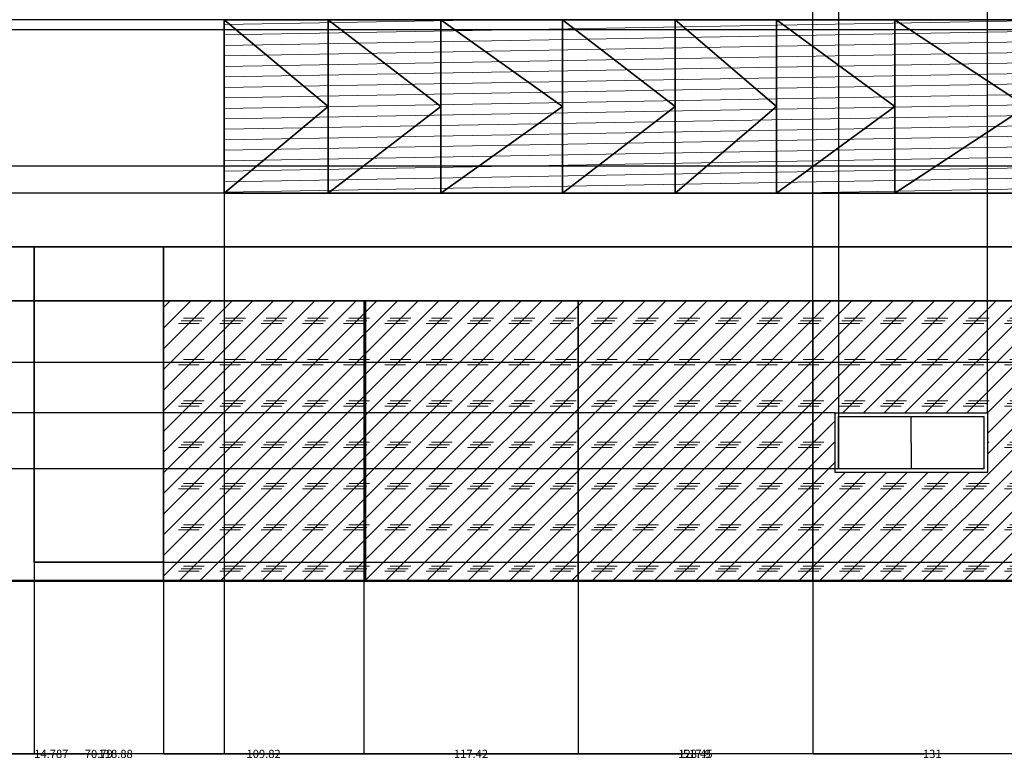
# Model space of a CAD drawing. Units: inches. Extents: x -1308 to 780, y 304 to 1023.
# Tile 5 of 7: x -138 to 402, y 304 to 709. Entities that reach past the tile are written whole.
import ezdxf

# ---------------------------------------------------------------- set-up
doc = ezdxf.new("R2010")
doc.units = ezdxf.units.IN
doc.header["$MEASUREMENT"] = 0
for name, color, linetype, lineweight in [('A-ANNO-DIMS', 2, 'Continuous', 18), ('A-ELEV', 7, 'Continuous', 35), ('A-ELEV-GRND', 7, 'Continuous', 50), ('A-ELEV-PATT', 8, 'Continuous', 13), ('A-GLAZ', 4, 'Continuous', 25)]:
    doc.layers.add(name, color=color, linetype=linetype, lineweight=lineweight)
doc.styles.get("Standard").update_dxf_attribs({"font": 'arial.ttf'})
doc.dimstyles.get("Standard").update_dxf_attribs({"dimtxt": 4.5, "dimasz": 0.18, "dimexe": 0.18, "dimexo": 0.0625, "dimgap": 0.09, "dimtad": 0, "dimtih": 1, "dimtoh": 1, "dimdec": 4, "dimzin": 0, "dimdsep": 46, "dimlunit": 4, "dimtxsty": 'Standard', "dimcen": 0.09, "dimadec": 0, "dimazin": 0, "dimtfac": 1, "dimtdec": 4, "dimtofl": 0, "dimtmove": 0, "dimatfit": 3, "dimfxl": 1, "dimtolj": 1, "dimtzin": 0, "dimarcsym": 0})

# ---------------------------------------------------------------- blocks, each defined once
blk = doc.blocks.new('*D1')
at = {"layer": 'A-ANNO-DIMS', "color": 0, "lineweight": -2, "transparency": 16777216}
for p, q in [((-1203.52, 401.95), (-1203.52, 307.09)), ((676.16, 401.95), (676.16, 307.09)), ((-1203.34, 307.27), (-272.9, 307.27)), ((675.98, 307.27), (-254.46, 307.27))]:
    blk.add_line(p, q, dxfattribs=at)
at = {"layer": 'A-ANNO-DIMS', "color": 0, "transparency": 16777216}
for points in [[(-1203.34, 307.3), (-1203.34, 307.24), (-1203.52, 307.27)], [(675.98, 307.3), (675.98, 307.24), (676.16, 307.27)]]:
    blk.add_solid(points, dxfattribs=at)
at = {"layer": 'Defpoints', "color": 0, "transparency": 16777216}
for p in [(-1203.52, 402.02), (676.16, 402.02), (676.16, 307.27)]:
    blk.add_point(p, dxfattribs=at)
at = {"layer": 'A-ANNO-DIMS', "color": 0, "transparency": 16777216, "insert": (-263.68, 307.27), "char_height": 4.5, "attachment_point": 5}
blk.add_mtext('\\A1;1879.7', dxfattribs=at)
blk = doc.blocks.new('*D9')
at = {"layer": 'A-ANNO-DIMS', "color": 0, "lineweight": -2, "transparency": 16777216}
for p, q in [((-144.73, 555.46), (-144.73, 307.09)), ((-129.95, 555.46), (-129.95, 307.09)), ((-144.55, 307.27), (-130.13, 307.27)), ((-129.95, 307.27), (-129.77, 307.27))]:
    blk.add_line(p, q, dxfattribs=at)
at = {"layer": 'A-ANNO-DIMS', "color": 0, "transparency": 16777216}
for points in [[(-144.55, 307.3), (-144.55, 307.24), (-144.73, 307.27)], [(-130.13, 307.3), (-130.13, 307.24), (-129.95, 307.27)]]:
    blk.add_solid(points, dxfattribs=at)
at = {"layer": 'Defpoints', "color": 0, "transparency": 16777216}
for p in [(-144.73, 555.52), (-129.95, 555.52), (-129.95, 307.27)]:
    blk.add_point(p, dxfattribs=at)
at = {"layer": 'A-ANNO-DIMS', "color": 0, "transparency": 16777216, "insert": (-120.55, 307.27), "char_height": 4.5, "attachment_point": 5}
blk.add_mtext('\\A1;14.787', dxfattribs=at)
blk = doc.blocks.new('*D10')
at = {"layer": 'A-ANNO-DIMS', "color": 0, "lineweight": -2, "transparency": 16777216}
for p, q in [((-129.95, 555.46), (-129.95, 307.09)), ((-59.16, 555.46), (-59.16, 307.09)), ((-129.77, 307.27), (-102.22, 307.27)), ((-59.34, 307.27), (-86.88, 307.27))]:
    blk.add_line(p, q, dxfattribs=at)
at = {"layer": 'A-ANNO-DIMS', "color": 0, "transparency": 16777216}
for points in [[(-129.77, 307.3), (-129.77, 307.24), (-129.95, 307.27)], [(-59.34, 307.3), (-59.34, 307.24), (-59.16, 307.27)]]:
    blk.add_solid(points, dxfattribs=at)
at = {"layer": 'Defpoints', "color": 0, "transparency": 16777216}
for p in [(-129.95, 555.52), (-59.16, 555.52), (-59.16, 307.27)]:
    blk.add_point(p, dxfattribs=at)
at = {"layer": 'A-ANNO-DIMS', "color": 0, "transparency": 16777216, "insert": (-94.55, 307.27), "char_height": 4.5, "attachment_point": 5}
blk.add_mtext('\\A1;70.79', dxfattribs=at)
blk = doc.blocks.new('*D11')
at = {"layer": 'A-ANNO-DIMS', "color": 0, "lineweight": -2, "transparency": 16777216}
for p, q in [((-59.16, 555.46), (-59.16, 307.09)), ((50.66, 555.46), (50.66, 307.09)), ((-58.98, 307.27), (-13.44, 307.27)), ((50.48, 307.27), (4.95, 307.27))]:
    blk.add_line(p, q, dxfattribs=at)
at = {"layer": 'A-ANNO-DIMS', "color": 0, "transparency": 16777216}
for points in [[(-58.98, 307.3), (-58.98, 307.24), (-59.16, 307.27)], [(50.48, 307.3), (50.48, 307.24), (50.66, 307.27)]]:
    blk.add_solid(points, dxfattribs=at)
at = {"layer": 'Defpoints', "color": 0, "transparency": 16777216}
for p in [(-59.16, 555.52), (50.66, 555.52), (50.66, 307.27)]:
    blk.add_point(p, dxfattribs=at)
at = {"layer": 'A-ANNO-DIMS', "color": 0, "transparency": 16777216, "insert": (-4.25, 307.27), "char_height": 4.5, "attachment_point": 5}
blk.add_mtext('\\A1;109.82', dxfattribs=at)
blk = doc.blocks.new('*D12')
at = {"layer": 'A-ANNO-DIMS', "color": 0, "lineweight": -2, "transparency": 16777216}
for p, q in [((50.66, 555.46), (50.66, 307.09)), ((168.08, 555.46), (168.08, 307.09)), ((50.84, 307.27), (100.18, 307.27)), ((167.9, 307.27), (118.57, 307.27))]:
    blk.add_line(p, q, dxfattribs=at)
at = {"layer": 'A-ANNO-DIMS', "color": 0, "transparency": 16777216}
for points in [[(50.84, 307.3), (50.84, 307.24), (50.66, 307.27)], [(167.9, 307.3), (167.9, 307.24), (168.08, 307.27)]]:
    blk.add_solid(points, dxfattribs=at)
at = {"layer": 'Defpoints', "color": 0, "transparency": 16777216}
for p in [(50.66, 555.52), (168.08, 555.52), (168.08, 307.27)]:
    blk.add_point(p, dxfattribs=at)
at = {"layer": 'A-ANNO-DIMS', "color": 0, "transparency": 16777216, "insert": (109.37, 307.27), "char_height": 4.5, "attachment_point": 5}
blk.add_mtext('\\A1;117.42', dxfattribs=at)
blk = doc.blocks.new('*D13')
at = {"layer": 'A-ANNO-DIMS', "color": 0, "lineweight": -2, "transparency": 16777216}
for p, q in [((168.08, 555.46), (168.08, 307.09)), ((296.53, 555.46), (296.53, 307.09)), ((168.26, 307.27), (223.07, 307.27)), ((296.35, 307.27), (241.54, 307.27))]:
    blk.add_line(p, q, dxfattribs=at)
at = {"layer": 'A-ANNO-DIMS', "color": 0, "transparency": 16777216}
for points in [[(168.26, 307.3), (168.26, 307.24), (168.08, 307.27)], [(296.35, 307.3), (296.35, 307.24), (296.53, 307.27)]]:
    blk.add_solid(points, dxfattribs=at)
at = {"layer": 'Defpoints', "color": 0, "transparency": 16777216}
for p in [(168.08, 555.52), (296.53, 555.52), (296.53, 307.27)]:
    blk.add_point(p, dxfattribs=at)
at = {"layer": 'A-ANNO-DIMS', "color": 0, "transparency": 16777216, "insert": (232.31, 307.27), "char_height": 4.5, "attachment_point": 5}
blk.add_mtext('\\A1;128.45', dxfattribs=at)
blk = doc.blocks.new('*D14')
at = {"layer": 'A-ANNO-DIMS', "color": 0, "lineweight": -2, "transparency": 16777216}
for p, q in [((296.53, 555.46), (296.53, 307.09)), ((427.54, 555.46), (427.54, 307.09)), ((296.71, 307.27), (357.62, 307.27)), ((427.36, 307.27), (366.45, 307.27))]:
    blk.add_line(p, q, dxfattribs=at)
at = {"layer": 'A-ANNO-DIMS', "color": 0, "transparency": 16777216}
for points in [[(296.71, 307.3), (296.71, 307.24), (296.53, 307.27)], [(427.36, 307.3), (427.36, 307.24), (427.54, 307.27)]]:
    blk.add_solid(points, dxfattribs=at)
at = {"layer": 'Defpoints', "color": 0, "transparency": 16777216}
for p in [(296.53, 555.52), (427.54, 555.52), (427.54, 307.27)]:
    blk.add_point(p, dxfattribs=at)
at = {"layer": 'A-ANNO-DIMS', "color": 0, "transparency": 16777216, "insert": (362.03, 307.27), "char_height": 4.5, "attachment_point": 5}
blk.add_mtext('\\A1;131', dxfattribs=at)
blk = doc.blocks.new('*D45')
at = {"layer": 'A-ANNO-DIMS', "color": 0, "lineweight": -2, "transparency": 16777216}
for p, q in [((-25.86, 614.44), (-25.86, 307.09)), ((-144.73, 584.98), (-144.73, 307.09)), ((-144.55, 307.27), (-94.52, 307.27)), ((-26.04, 307.27), (-76.07, 307.27))]:
    blk.add_line(p, q, dxfattribs=at)
at = {"layer": 'A-ANNO-DIMS', "color": 0, "transparency": 16777216}
for points in [[(-144.55, 307.3), (-144.55, 307.24), (-144.73, 307.27)], [(-26.04, 307.3), (-26.04, 307.24), (-25.86, 307.27)]]:
    blk.add_solid(points, dxfattribs=at)
at = {"layer": 'Defpoints', "color": 0, "transparency": 16777216}
for p in [(-25.86, 614.51), (-144.73, 585.04), (-25.86, 307.27)]:
    blk.add_point(p, dxfattribs=at)
at = {"layer": 'A-ANNO-DIMS', "color": 0, "transparency": 16777216, "insert": (-85.3, 307.27), "char_height": 4.5, "attachment_point": 5}
blk.add_mtext('\\A1;118.88', dxfattribs=at)
blk = doc.blocks.new('*D46')
at = {"layer": 'A-ANNO-DIMS', "color": 0, "lineweight": -2, "transparency": 16777216}
for p, q in [((-25.86, 614.44), (-25.86, 307.09)), ((492.05, 614.44), (492.05, 307.09)), ((-25.68, 307.27), (225.41, 307.27)), ((491.87, 307.27), (240.78, 307.27))]:
    blk.add_line(p, q, dxfattribs=at)
at = {"layer": 'A-ANNO-DIMS', "color": 0, "transparency": 16777216}
for points in [[(-25.68, 307.3), (-25.68, 307.24), (-25.86, 307.27)], [(491.87, 307.3), (491.87, 307.24), (492.05, 307.27)]]:
    blk.add_solid(points, dxfattribs=at)
at = {"layer": 'Defpoints', "color": 0, "transparency": 16777216}
for p in [(-25.86, 614.51), (492.05, 614.51), (492.05, 307.27)]:
    blk.add_point(p, dxfattribs=at)
at = {"layer": 'A-ANNO-DIMS', "color": 0, "transparency": 16777216, "insert": (233.1, 307.27), "char_height": 4.5, "attachment_point": 5}
blk.add_mtext('\\A1;517.9', dxfattribs=at)
blk = doc.blocks.new('*D55')
at = {"layer": 'A-ANNO-DIMS', "color": 0, "lineweight": -2, "transparency": 16777216}
for p, q in [((310.77, 463.5), (310.77, 1019.77)), ((310.95, 1019.59), (343.86, 1019.59)), ((392.14, 1019.59), (359.23, 1019.59)), ((392.32, 494.13), (392.32, 1019.77))]:
    blk.add_line(p, q, dxfattribs=at)
at = {"layer": 'A-ANNO-DIMS', "color": 0, "transparency": 16777216}
for points in [[(310.95, 1019.62), (310.95, 1019.56), (310.77, 1019.59)], [(392.14, 1019.62), (392.14, 1019.56), (392.32, 1019.59)]]:
    blk.add_solid(points, dxfattribs=at)
at = {"layer": 'Defpoints', "color": 0, "transparency": 16777216}
for p in [(392.32, 1019.59), (392.32, 494.07), (310.77, 463.43)]:
    blk.add_point(p, dxfattribs=at)
at = {"layer": 'A-ANNO-DIMS', "color": 0, "transparency": 16777216, "insert": (351.54, 1019.59), "char_height": 4.5, "attachment_point": 5}
blk.add_mtext('\\A1;81.56', dxfattribs=at)
blk = doc.blocks.new('*D56')
at = {"layer": 'A-ANNO-DIMS', "color": 0, "lineweight": -2, "transparency": 16777216}
for p, q in [((296.53, 402.08), (296.53, 1019.77)), ((296.71, 1019.59), (310.59, 1019.59)), ((310.77, 463.5), (310.77, 1019.77)), ((310.77, 1019.59), (310.95, 1019.59))]:
    blk.add_line(p, q, dxfattribs=at)
at = {"layer": 'A-ANNO-DIMS', "color": 0, "transparency": 16777216}
for points in [[(296.71, 1019.62), (296.71, 1019.56), (296.53, 1019.59)], [(310.59, 1019.62), (310.59, 1019.56), (310.77, 1019.59)]]:
    blk.add_solid(points, dxfattribs=at)
at = {"layer": 'Defpoints', "color": 0, "transparency": 16777216}
for p in [(310.77, 1019.59), (310.77, 463.43), (296.53, 402.02)]:
    blk.add_point(p, dxfattribs=at)
at = {"layer": 'A-ANNO-DIMS', "color": 0, "transparency": 16777216, "insert": (320.15, 1019.59), "char_height": 4.5, "attachment_point": 5}
blk.add_mtext('\\A1;14.234', dxfattribs=at)
blk = doc.blocks.new('*D58')
at = {"layer": 'A-ANNO-DIMS', "color": 0, "lineweight": -2, "transparency": 16777216}
for p, q in [((-1187.44, 521.84), (771.09, 521.84)), ((770.91, 521.66), (770.91, 464.32)), ((770.91, 402.2), (770.91, 459.54)), ((-1187.44, 402.02), (771.09, 402.02))]:
    blk.add_line(p, q, dxfattribs=at)
at = {"layer": 'A-ANNO-DIMS', "color": 0, "transparency": 16777216}
for points in [[(770.88, 521.66), (770.94, 521.66), (770.91, 521.84)], [(770.88, 402.2), (770.94, 402.2), (770.91, 402.02)]]:
    blk.add_solid(points, dxfattribs=at)
at = {"layer": 'Defpoints', "color": 0, "transparency": 16777216}
for p in [(-1187.5, 521.84), (770.91, 521.84), (-1187.5, 402.02)]:
    blk.add_point(p, dxfattribs=at)
at = {"layer": 'A-ANNO-DIMS', "color": 0, "transparency": 16777216, "insert": (770.91, 461.93), "char_height": 4.5, "attachment_point": 5}
blk.add_mtext('\\A1;119.83', dxfattribs=at)
blk = doc.blocks.new('*D63')
at = {"layer": 'A-ANNO-DIMS', "color": 0, "lineweight": -2, "transparency": 16777216}
for p, q in [((-843.54, 629.44), (771.09, 629.44)), ((770.91, 629.26), (770.91, 518.12)), ((770.91, 402.2), (770.91, 513.34)), ((-843.54, 402.02), (771.09, 402.02))]:
    blk.add_line(p, q, dxfattribs=at)
at = {"layer": 'A-ANNO-DIMS', "color": 0, "transparency": 16777216}
for points in [[(770.88, 629.26), (770.94, 629.26), (770.91, 629.44)], [(770.88, 402.2), (770.94, 402.2), (770.91, 402.02)]]:
    blk.add_solid(points, dxfattribs=at)
at = {"layer": 'Defpoints', "color": 0, "transparency": 16777216}
for p in [(-843.6, 629.44), (770.91, 629.44), (-843.6, 402.02)]:
    blk.add_point(p, dxfattribs=at)
at = {"layer": 'A-ANNO-DIMS', "color": 0, "transparency": 16777216, "insert": (770.91, 515.73), "char_height": 4.5, "attachment_point": 5}
blk.add_mtext('\\A1;227.43', dxfattribs=at)
blk = doc.blocks.new('*D64')
at = {"layer": 'A-ANNO-DIMS', "color": 0, "lineweight": -2, "transparency": 16777216}
for p, q in [((-843.54, 704.09), (771.09, 704.09)), ((770.91, 703.91), (770.91, 669.15)), ((770.91, 629.62), (770.91, 664.38)), ((-843.54, 629.44), (771.09, 629.44))]:
    blk.add_line(p, q, dxfattribs=at)
at = {"layer": 'A-ANNO-DIMS', "color": 0, "transparency": 16777216}
for points in [[(770.88, 703.91), (770.94, 703.91), (770.91, 704.09)], [(770.88, 629.62), (770.94, 629.62), (770.91, 629.44)]]:
    blk.add_solid(points, dxfattribs=at)
at = {"layer": 'Defpoints', "color": 0, "transparency": 16777216}
for p in [(-843.6, 704.09), (770.91, 704.09), (-843.6, 629.44)]:
    blk.add_point(p, dxfattribs=at)
at = {"layer": 'A-ANNO-DIMS', "color": 0, "transparency": 16777216, "insert": (770.91, 666.76), "char_height": 4.5, "attachment_point": 5}
blk.add_mtext('\\A1;74.64', dxfattribs=at)
blk = doc.blocks.new('*D65')
at = {"layer": 'A-ANNO-DIMS', "color": 0, "lineweight": -2, "transparency": 16777216}
for p, q in [((-843.54, 753.04), (771.09, 753.04)), ((770.91, 752.86), (770.91, 730.95)), ((770.91, 704.27), (770.91, 726.17)), ((-843.54, 704.09), (771.09, 704.09))]:
    blk.add_line(p, q, dxfattribs=at)
at = {"layer": 'A-ANNO-DIMS', "color": 0, "transparency": 16777216}
for points in [[(770.88, 752.86), (770.94, 752.86), (770.91, 753.04)], [(770.88, 704.27), (770.94, 704.27), (770.91, 704.09)]]:
    blk.add_solid(points, dxfattribs=at)
at = {"layer": 'Defpoints', "color": 0, "transparency": 16777216}
for p in [(-843.6, 753.04), (770.91, 753.04), (-843.6, 704.09)]:
    blk.add_point(p, dxfattribs=at)
at = {"layer": 'A-ANNO-DIMS', "color": 0, "transparency": 16777216, "insert": (770.91, 728.56), "char_height": 4.5, "attachment_point": 5}
blk.add_mtext('\\A1;48.95', dxfattribs=at)
blk = doc.blocks.new('*D78')
at = {"layer": 'A-ANNO-DIMS', "color": 0, "lineweight": -2, "transparency": 16777216}
for p, q in [((-129.88, 585.04), (771.09, 585.04)), ((770.91, 584.86), (770.91, 501.1)), ((770.91, 412.56), (770.91, 496.32)), ((-129.88, 412.38), (771.09, 412.38))]:
    blk.add_line(p, q, dxfattribs=at)
at = {"layer": 'A-ANNO-DIMS', "color": 0, "transparency": 16777216}
for points in [[(770.88, 584.86), (770.94, 584.86), (770.91, 585.04)], [(770.88, 412.56), (770.94, 412.56), (770.91, 412.38)]]:
    blk.add_solid(points, dxfattribs=at)
at = {"layer": 'Defpoints', "color": 0, "transparency": 16777216}
for p in [(-129.95, 585.04), (770.91, 585.04), (-129.95, 412.38)]:
    blk.add_point(p, dxfattribs=at)
at = {"layer": 'A-ANNO-DIMS', "color": 0, "transparency": 16777216, "insert": (770.91, 498.71), "char_height": 4.5, "attachment_point": 5}
blk.add_mtext('\\A1;172.66', dxfattribs=at)
blk = doc.blocks.new('*D79')
at = {"layer": 'A-ANNO-DIMS', "color": 0, "lineweight": -2, "transparency": 16777216}
for p, q in [((310.7, 463.43), (-1298.45, 463.43)), ((-1298.27, 463.25), (-1298.27, 435.11)), ((-1298.27, 402.2), (-1298.27, 430.34)), ((296.47, 402.02), (-1298.45, 402.02))]:
    blk.add_line(p, q, dxfattribs=at)
at = {"layer": 'A-ANNO-DIMS', "color": 0, "transparency": 16777216}
for points in [[(-1298.3, 463.25), (-1298.24, 463.25), (-1298.27, 463.43)], [(-1298.3, 402.2), (-1298.24, 402.2), (-1298.27, 402.02)]]:
    blk.add_solid(points, dxfattribs=at)
at = {"layer": 'Defpoints', "color": 0, "transparency": 16777216}
for p in [(-1298.27, 463.43), (310.77, 463.43), (296.53, 402.02)]:
    blk.add_point(p, dxfattribs=at)
at = {"layer": 'A-ANNO-DIMS', "color": 0, "transparency": 16777216, "insert": (-1298.27, 432.72), "char_height": 4.5, "attachment_point": 5}
blk.add_mtext('\\A1;61.42', dxfattribs=at)
blk = doc.blocks.new('*D80')
at = {"layer": 'A-ANNO-DIMS', "color": 0, "lineweight": -2, "transparency": 16777216}
for p, q in [((308.7, 494.07), (-1298.45, 494.07)), ((-1298.27, 493.89), (-1298.27, 481.14)), ((-1298.27, 463.61), (-1298.27, 476.36)), ((310.7, 463.43), (-1298.45, 463.43))]:
    blk.add_line(p, q, dxfattribs=at)
at = {"layer": 'A-ANNO-DIMS', "color": 0, "transparency": 16777216}
for points in [[(-1298.3, 493.89), (-1298.24, 493.89), (-1298.27, 494.07)], [(-1298.3, 463.61), (-1298.24, 463.61), (-1298.27, 463.43)]]:
    blk.add_solid(points, dxfattribs=at)
at = {"layer": 'Defpoints', "color": 0, "transparency": 16777216}
for p in [(-1298.27, 494.07), (308.77, 494.07), (310.77, 463.43)]:
    blk.add_point(p, dxfattribs=at)
at = {"layer": 'A-ANNO-DIMS', "color": 0, "transparency": 16777216, "insert": (-1298.27, 478.75), "char_height": 4.5, "attachment_point": 5}
blk.add_mtext('\\A1;30.64', dxfattribs=at)
blk = doc.blocks.new('*D81')
at = {"layer": 'A-ANNO-DIMS', "color": 0, "lineweight": -2, "transparency": 16777216}
for p, q in [((-25.92, 614.51), (-1298.45, 614.51)), ((-1298.27, 614.33), (-1298.27, 602.16)), ((-1298.27, 585.22), (-1298.27, 597.39)), ((-59.22, 585.04), (-1298.45, 585.04))]:
    blk.add_line(p, q, dxfattribs=at)
at = {"layer": 'A-ANNO-DIMS', "color": 0, "transparency": 16777216}
for points in [[(-1298.3, 614.33), (-1298.24, 614.33), (-1298.27, 614.51)], [(-1298.3, 585.22), (-1298.24, 585.22), (-1298.27, 585.04)]]:
    blk.add_solid(points, dxfattribs=at)
at = {"layer": 'Defpoints', "color": 0, "transparency": 16777216}
for p in [(-1298.27, 614.51), (-25.86, 614.51), (-59.16, 585.04)]:
    blk.add_point(p, dxfattribs=at)
at = {"layer": 'A-ANNO-DIMS', "color": 0, "transparency": 16777216, "insert": (-1298.27, 599.77), "char_height": 4.5, "attachment_point": 5}
blk.add_mtext('\\A1;29.47', dxfattribs=at)
blk = doc.blocks.new('*D82')
at = {"layer": 'A-ANNO-DIMS', "color": 0, "lineweight": -2, "transparency": 16777216}
for p, q in [((-25.92, 709.46), (-1298.45, 709.46)), ((-1298.27, 709.28), (-1298.27, 664.37)), ((-1298.27, 614.69), (-1298.27, 659.6)), ((-25.92, 614.51), (-1298.45, 614.51))]:
    blk.add_line(p, q, dxfattribs=at)
at = {"layer": 'A-ANNO-DIMS', "color": 0, "transparency": 16777216}
for points in [[(-1298.3, 709.28), (-1298.24, 709.28), (-1298.27, 709.46)], [(-1298.3, 614.69), (-1298.24, 614.69), (-1298.27, 614.51)]]:
    blk.add_solid(points, dxfattribs=at)
at = {"layer": 'Defpoints', "color": 0, "transparency": 16777216}
for p in [(-1298.27, 709.46), (-25.86, 709.46), (-25.86, 614.51)]:
    blk.add_point(p, dxfattribs=at)
at = {"layer": 'A-ANNO-DIMS', "color": 0, "transparency": 16777216, "insert": (-1298.27, 661.98), "char_height": 4.5, "attachment_point": 5}
blk.add_mtext('\\A1;94.95', dxfattribs=at)

msp = doc.modelspace()

# ---------------------------------------------------------------- hatches: boundary and pattern name
at = {"layer": 'A-ELEV-PATT'}
h = msp.add_hatch(dxfattribs=at)
h.set_pattern_fill('ANSI31', color=256, scale=46, angle=136)
h.paths.add_polyline_path([(-25.8575, 709.4602), (-25.8575, 614.5069), (31.1601, 661.9835)])
h.paths.add_polyline_path([(31.1601, 709.4602), (-25.8575, 709.4602), (31.1601, 661.9835)], flags=17)
h.paths.add_polyline_path([(31.1601, 661.9835), (-25.8575, 614.5069), (31.1601, 614.5069)])
h.paths.add_polyline_path([(92.9293, 709.4602), (31.1601, 709.4602), (92.9293, 661.9835)])
h.paths.add_polyline_path([(31.1601, 709.4602), (31.1601, 661.9835), (31.1601, 614.5069), (92.9293, 661.9835)])
h.paths.add_polyline_path([(92.9293, 661.9835), (31.1601, 614.5069), (92.9293, 614.5069)])
h.paths.add_polyline_path([(159.4499, 661.9835), (92.9293, 709.4602), (92.9293, 661.9835), (92.9293, 614.5069)])
h.paths.add_polyline_path([(159.4499, 661.9835), (92.9293, 614.5069), (159.4499, 614.5069)])
h.paths.add_polyline_path([(159.4499, 709.4602), (92.9293, 709.4602), (159.4499, 661.9835)], flags=17)
h.paths.add_polyline_path([(159.4499, 709.4602), (159.4499, 614.5069), (221.219, 661.9835)])
h.paths.add_polyline_path([(221.219, 709.4602), (159.4499, 709.4602), (221.219, 661.9835)])
h.paths.add_polyline_path([(221.219, 661.9835), (159.4499, 614.5069), (221.219, 614.5069)])
h.paths.add_polyline_path([(276.6529, 661.9835), (221.219, 709.4602), (221.219, 661.9835), (221.219, 614.5069)])
h.paths.add_polyline_path([(276.6529, 661.9835), (221.219, 614.5069), (276.6529, 614.5069)])
h.paths.add_polyline_path([(276.6529, 709.4602), (221.219, 709.4602), (276.6529, 661.9835)])
h.paths.add_polyline_path([(341.5897, 661.9835), (276.6529, 709.4602), (276.6529, 661.9835), (276.6529, 614.5069)])
h.paths.add_polyline_path([(341.5897, 709.4602), (276.6529, 709.4602), (341.5897, 661.9835)])
h.paths.add_polyline_path([(341.5897, 661.9835), (276.6529, 614.5069), (341.5897, 614.5069)])
h.paths.add_polyline_path([(413.6537, 661.9835), (341.5897, 709.4602), (341.5897, 661.9835), (341.5897, 614.5069)])
h.paths.add_polyline_path([(413.6537, 661.9835), (341.5897, 614.5069), (413.6537, 614.5069)])
h.paths.add_polyline_path([(492.0529, 661.9835), (413.6537, 709.4602), (413.6537, 614.5069)])
h.paths.add_polyline_path([(492.0529, 661.9835), (413.6537, 614.5069), (492.0529, 614.5069)])
h.paths.add_polyline_path([(492.0529, 709.4602), (413.6537, 709.4602), (492.0529, 661.9835)], flags=17)
h.paths.add_polyline_path([(413.6537, 709.4602), (341.5897, 709.4602), (413.6537, 661.9835)])
h = msp.add_hatch(dxfattribs=at)
h.set_pattern_fill('CORK', color=256, scale=64, angle=45)
h.set_pattern_definition([(45, (0, 0), (-5.656854, 5.656854), []), (180, (5.657, 0), (-2e-15, -22.6274), [11.3137, -11.3137]), (180, (7.07, 1.414), (-2e-15, -22.6274), [11.3137, -11.3137]), (180, (8.485, 2.828), (-2e-15, -22.6274), [11.3137, -11.3137])])
h.paths.add_polyline_path([(51.6368, 555.5236), (50.6624, 555.5236), (-59.1597, 555.5236), (-59.1597, 402.0158), (47.1224, 402.0158), (51.6368, 402.0158)])
h.paths.add_polyline_path([(168.0796, 555.5236), (51.6368, 555.5236), (51.6368, 402.0158), (168.0796, 402.0158)])
h.paths.add_polyline_path([(296.5309, 555.5236), (168.0796, 555.5236), (168.0796, 402.0158), (296.5309, 402.0158)])
h.paths.add_polyline_path([(427.5353, 555.5236), (296.5309, 555.5236), (296.5309, 402.0158), (427.5353, 402.0158)])
h.paths.add_polyline_path([(308.7651, 461.4331), (308.7651, 494.0703), (392.3226, 494.0703), (392.3226, 461.4331)], flags=16)
h.paths.add_polyline_path([(310.7651, 463.4331), (310.7651, 492.0703), (390.3226, 492.0703), (390.3226, 463.4331)], flags=0)
h.paths.add_polyline_path([(551.6272, 555.5236), (427.5353, 555.5236), (427.5353, 402.0158), (551.6272, 402.0158)])
h.paths.add_polyline_path([(676.1576, 555.5236), (551.6272, 555.5236), (551.6272, 402.0158), (676.1576, 402.0158), (676.1576, 462.0158)])

# ---------------------------------------------------------------- linework, layer by layer
at = {"layer": 'A-ELEV'}
for p, q in [((-25.8575, 709.4602), (31.1601, 661.9835)), ((31.1601, 709.4602), (31.1601, 614.5069)), ((31.1601, 709.4602), (92.9293, 661.9835)), ((92.9293, 709.4602), (92.9293, 614.5069)), ((92.9293, 709.4602), (159.4499, 661.9835)), ((159.4499, 709.4602), (159.4499, 614.5069)), ((159.4499, 709.4602), (221.219, 661.9835)), ((221.219, 709.4602), (221.219, 614.5069)), ((221.219, 709.4602), (276.6529, 661.9835)), ((276.6529, 709.4602), (276.6529, 614.5069)), ((276.6529, 709.4602), (341.5897, 661.9835)), ((341.5897, 709.4602), (341.5897, 614.5069)), ((341.5897, 709.4602), (413.6537, 661.9835)), ((31.1601, 661.9835), (-25.8575, 614.5069)), ((92.9293, 661.9835), (31.1601, 614.5069)), ((159.4499, 661.9835), (92.9293, 614.5069)), ((221.219, 661.9835), (159.4499, 614.5069)), ((276.6529, 661.9835), (221.219, 614.5069)), ((341.5897, 661.9835), (276.6529, 614.5069)), ((413.6537, 661.9835), (341.5897, 614.5069)), ((-144.7329, 585.0385), (526.9606, 585.0385)), ((-129.9455, 555.5236), (-129.9455, 585.0385)), ((-59.1597, 555.5236), (-59.1597, 585.0385)), ((50.6624, 555.5236), (-144.7329, 555.5236)), ((-129.9455, 412.3765), (-129.9455, 555.5236)), ((-59.1597, 555.5236), (-59.1597, 402.0158)), ((676.1576, 555.5236), (50.6624, 555.5236)), ((51.6368, 555.5236), (51.6368, 402.0158)), ((168.0796, 555.5236), (168.0796, 402.0158)), ((296.5309, 555.5236), (296.5309, 402.0158)), ((-59.1597, 412.3765), (-129.9455, 412.3765))]:
    msp.add_line(p, q, dxfattribs=at)
msp.add_lwpolyline([(-25.8575, 709.4602), (492.0529, 709.4602), (492.0529, 614.5069), (-25.8575, 614.5069)], close=True, dxfattribs=at)
at = {"layer": 'A-ELEV-GRND'}
for q in [(-144.7329, 402.0158), (676.1576, 402.0158)]:
    msp.add_line((47.1224, 402.0158), q, dxfattribs=at)
at = {"layer": 'A-GLAZ'}
for q in [(350.5439, 492.0703), (350.5439, 463.4331)]:
    msp.add_line((350.5439, 477.7517), q, dxfattribs=at)
for points in [[(308.7651, 494.0703), (392.3226, 494.0703), (392.3226, 461.4331), (308.7651, 461.4331)], [(310.7651, 492.0703), (390.3226, 492.0703), (390.3226, 463.4331), (310.7651, 463.4331)]]:
    msp.add_lwpolyline(points, close=True, dxfattribs=at)

# ---------------------------------------------------------------- dimensions: what is measured, and where the dimension line sits
at = {"layer": 'A-ANNO-DIMS'}
for base, p1, p2, override, picture, middle in [((310.7651, 1019.5921), (296.5309, 402.0158), (310.7651, 463.4331), {"dimdec": 3, "dimlfac": 1, "dimrnd": 0, "dimzin": 0, "dimdsep": 46, "dimlunit": 2}, '*D56', (320.1548, 1019.5921)), ((392.3226, 1019.5921), (310.7651, 463.4331), (392.3226, 494.0703), {"dimdec": 2, "dimlfac": 1, "dimrnd": 0, "dimzin": 0, "dimdsep": 46, "dimlunit": 2}, '*D55', (351.5439, 1019.5921)), ((-25.8575, 307.2658), (-144.7329, 585.0385), (-25.8575, 614.5069), {"dimdec": 2, "dimlfac": 1, "dimrnd": 0, "dimzin": 0, "dimdsep": 46, "dimlunit": 2}, '*D45', (-85.2952, 307.2658)), ((492.0529, 307.2658), (-25.8575, 614.5069), (492.0529, 614.5069), {"dimdec": 1, "dimlfac": 1, "dimrnd": 0, "dimzin": 0, "dimdsep": 46, "dimlunit": 2}, '*D46', (233.0977, 307.2658)), ((-129.9455, 307.2658), (-144.7329, 555.5236), (-129.9455, 555.5236), {"dimdec": 3, "dimlfac": 1, "dimrnd": 0, "dimzin": 0, "dimdsep": 46, "dimlunit": 2}, '*D9', (-120.5466, 307.2658)), ((-59.1597, 307.2658), (-129.9455, 555.5236), (-59.1597, 555.5236), {"dimdec": 2, "dimlfac": 1, "dimrnd": 0, "dimzin": 0, "dimdsep": 46, "dimlunit": 2}, '*D10', (-94.5526, 307.2658)), ((50.6624, 307.2658), (-59.1597, 555.5236), (50.6624, 555.5236), {"dimdec": 2, "dimlfac": 1, "dimrnd": 0, "dimzin": 0, "dimdsep": 46, "dimlunit": 2}, '*D11', (-4.2486, 307.2658)), ((168.0796, 307.2658), (50.6624, 555.5236), (168.0796, 555.5236), {"dimdec": 2, "dimlfac": 1, "dimrnd": 0, "dimzin": 0, "dimdsep": 46, "dimlunit": 2}, '*D12', (109.371, 307.2658)), ((296.5309, 307.2658), (168.0796, 555.5236), (296.5309, 555.5236), {"dimdec": 2, "dimlfac": 1, "dimrnd": 0, "dimzin": 0, "dimdsep": 46, "dimlunit": 2}, '*D13', (232.3052, 307.2658)), ((427.5353, 307.2658), (296.5309, 555.5236), (427.5353, 555.5236), {"dimdec": 0, "dimlfac": 1, "dimrnd": 0, "dimzin": 0, "dimdsep": 46, "dimlunit": 2}, '*D14', (362.0331, 307.2658)), ((676.1576, 307.2658), (-1203.518, 402.0158), (676.1576, 402.0158), {"dimdec": 1, "dimlfac": 1, "dimrnd": 0, "dimzin": 0, "dimdsep": 46, "dimlunit": 2}, '*D1', (-263.6802, 307.2658))]:
    dim = msp.add_linear_dim(base=base, p1=p1, p2=p2, dimstyle='Standard', override=override, dxfattribs=at)
    dim.commit()
    dim.dimension.update_dxf_attribs({"geometry": picture, "text_midpoint": middle})
for base, p1, p2, picture, middle in [((770.9076, 753.0385), (-843.5988, 704.0857), (-843.5988, 753.0385), '*D65', (770.9076, 728.5621)), ((-1298.268, 709.4602), (-25.8575, 614.5069), (-25.8575, 709.4602), '*D82', (-1298.268, 661.9835)), ((770.9076, 704.0857), (-843.5988, 629.4421), (-843.5988, 704.0857), '*D64', (770.9076, 666.7639)), ((770.9076, 629.4421), (-843.5988, 402.0158), (-843.5988, 629.4421), '*D63', (770.9076, 515.729)), ((-1298.268, 614.5069), (-59.1597, 585.0385), (-25.8575, 614.5069), '*D81', (-1298.268, 599.7727)), ((770.9076, 585.0385), (-129.9455, 412.3765), (-129.9455, 585.0385), '*D78', (770.9076, 498.7075)), ((770.9076, 521.8442), (-1187.498, 402.0158), (-1187.498, 521.8442), '*D58', (770.9076, 461.93)), ((-1298.268, 494.0703), (310.7651, 463.4331), (308.7651, 494.0703), '*D80', (-1298.268, 478.7517)), ((-1298.268, 463.4331), (296.5309, 402.0158), (310.7651, 463.4331), '*D79', (-1298.268, 432.7245))]:
    dim = msp.add_linear_dim(base=base, p1=p1, p2=p2, angle=90, dimstyle='Standard', override={"dimdec": 2, "dimlfac": 1, "dimrnd": 0, "dimzin": 0, "dimdsep": 46, "dimlunit": 2}, dxfattribs=at)
    dim.commit()
    dim.dimension.update_dxf_attribs({"geometry": picture, "text_midpoint": middle})

doc.saveas('drawing.dxf')
